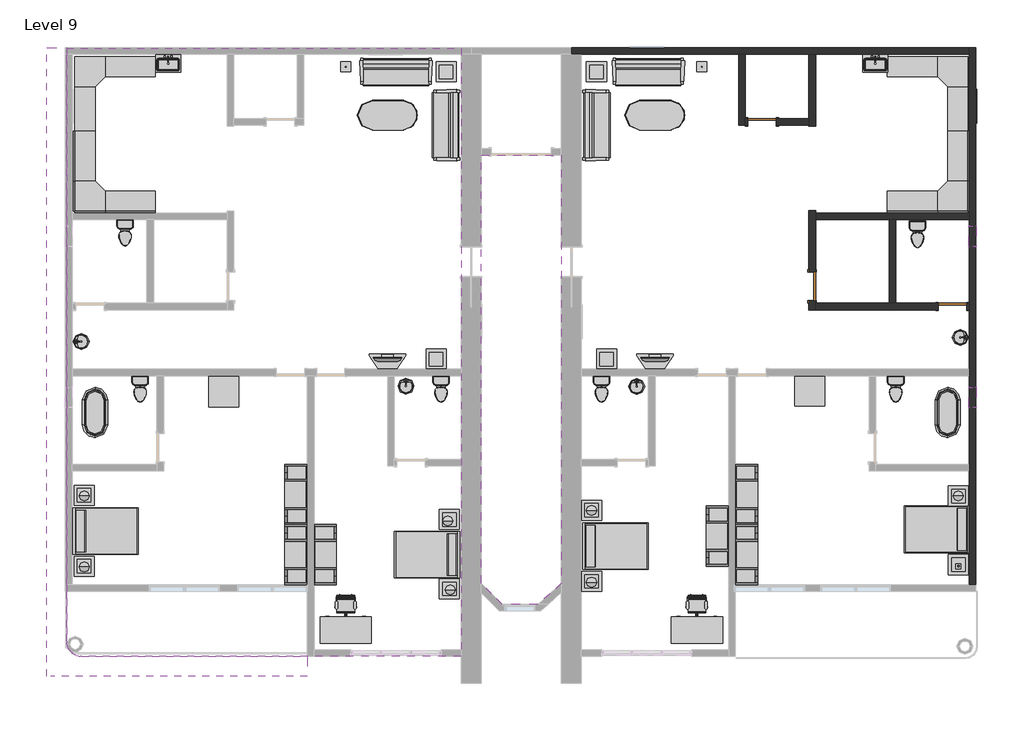
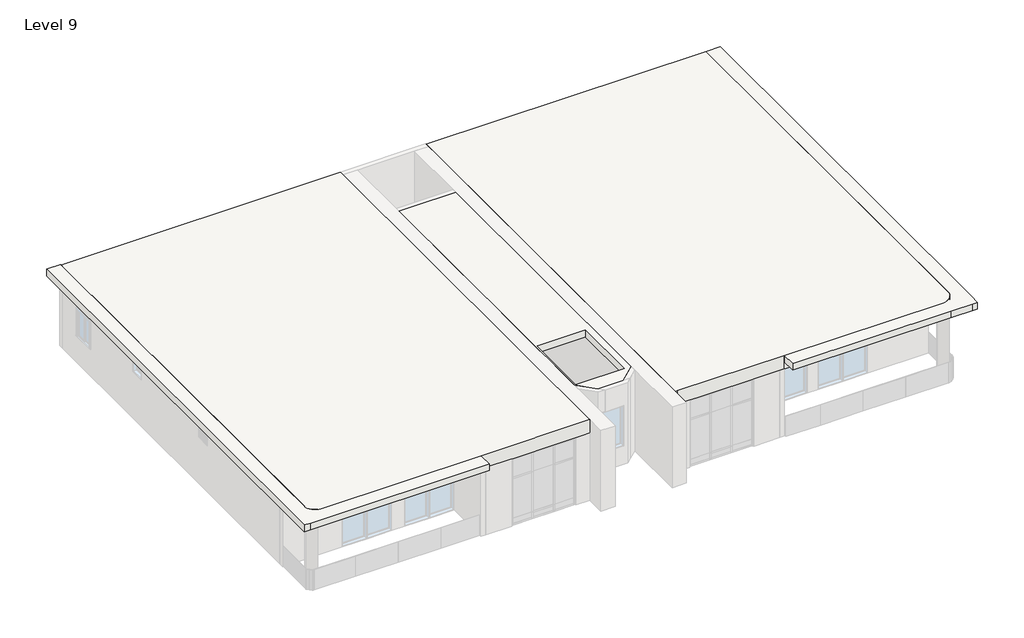
# One storey, part 3 of 3: 42 furniture elements, 14 flow terminals, 10 light fixtures, 9 walls, 3 doors, 3 slabs, 3 windows.
"""IFC4 building model written with IfcOpenShell, lengths in millimetres."""

from ifc_helpers import new_model, si_unit, point, frame, frame_2d, origin, place, context, project, spatial, polyline, circle_curve, trimmed, segment, composite_curve, outline, extrude, faceted_brep, transform, mapped, element, save
from components import door_2703ae13, door_10fd3a06, flow_terminal_38af2918, flow_terminal_d49f872f, toilet_domestic_3d_toilet_domestic_3d_f7549cf7, toilet_domestic_3d_toilet_domestic_3d_183bbd19, flow_terminal_b374fae2, furniture_07436f11, furniture_096e7f55, chair_task_arms_chair_task_arms_fa5a08ef, furniture_072f6425, furniture_cf0b6580, furniture_aff9b2fb, furniture_56245f3a, tv_stand_tv_stand_6ce107e5, furniture_b5c51a22, furniture_2c34a4f9, furniture_4d44e21c, furniture_45e3acac, light_fixture_100w_120v_8564026f, table_lamp_hemispheric_60w_120v_02721d88, window_0038ecf3, window_54100e87

model = new_model("IFC4")

# Units and contexts
model_context = context("Model", 3, world=origin())
ifc_project = project(units=[si_unit("LENGTHUNIT", "METRE", prefix="MILLI")], contexts=[model_context])

# Site, building, storey
site = spatial("IfcSite", under=ifc_project)
building = spatial("IfcBuilding", under=site)
storey = spatial("IfcBuildingStorey", under=building, Name="Level 9", Elevation=29260.8)

# Doors
placement = place(None, origin())
door_shape = door_2703ae13(model_context)
element("IfcDoor", 1, ObjectType="Door-Single-Panel.0001 : 34\" x 80\"", at=placement, inside=storey, context=model_context, shape_type="MappedRepresentation", body=[
    mapped(door_shape, transform((2522.0012296, 9464.0758558, 29260.8), x_axis=(-1.0, 0.0, 0.0), y_axis=(0.0, -1.0, 0.0), z_axis=(0.0, 0.0, 1.0))),
])
door_2_shape = door_10fd3a06(model_context)
element("IfcDoor", 2, ObjectType="Door-Single-Panel.0001 : 34\" x 80\"", at=placement, inside=storey, context=model_context, shape_type="MappedRepresentation", body=[
    mapped(door_2_shape, transform((8313.2012296, 3850.6758558, 29260.8), x_axis=(1.0, 0.0, 0.0), y_axis=(0.0, 1.0, 0.0), z_axis=(0.0, 0.0, 1.0))),
])
element("IfcDoor", 3, ObjectType="Door-Single-Panel.0001 : 34\" x 80\"", at=placement, inside=storey, context=model_context, shape_type="MappedRepresentation", body=[
    mapped(door_2_shape, transform((4046.0012296, 4460.2758558, 29260.8), x_axis=(0.0, -1.0, 0.0), y_axis=(1.0, 0.0, 0.0), z_axis=(0.0, 0.0, 1.0))),
])

# Flow terminals
flow_terminal_shape = flow_terminal_38af2918(model_context)
element("IfcFlowTerminal", 4, ObjectType="Sink Kitchen-Single : 30\" x 21\"", at=placement, inside=storey, context=model_context, shape_type="MappedRepresentation", body=[
    mapped(flow_terminal_shape, transform((-15540.388011, 11239.7304546, 29260.8), x_axis=(1.0, 0.0, 0.0), y_axis=(0.0, 1.0, 0.0), z_axis=(0.0, 0.0, 1.0))),
])
element("IfcFlowTerminal", 5, ObjectType="Sink Kitchen-Single : 30\" x 21\"", at=placement, inside=storey, context=model_context, shape_type="MappedRepresentation", body=[
    mapped(flow_terminal_shape, transform((5948.011989, 11239.7304546, 29260.8), x_axis=(1.0, 0.0, 0.0), y_axis=(0.0, 1.0, 0.0), z_axis=(0.0, 0.0, 1.0))),
])
flow_terminal_2_shape = flow_terminal_d49f872f(model_context)
element("IfcFlowTerminal", 6, ObjectType="Sink Vanity-Round : 19\" x 19\"", at=placement, inside=storey, context=model_context, shape_type="MappedRepresentation", body=[
    mapped(flow_terminal_2_shape, transform((-18084.6070794, 2687.2241152, 29260.8), x_axis=(0.0, 1.0, 0.0), y_axis=(-1.0, 0.0, 0.0), z_axis=(0.0, 0.0, 1.0))),
])
element("IfcFlowTerminal", 7, ObjectType="Sink Vanity-Round : 19\" x 19\"", at=placement, inside=storey, context=model_context, shape_type="MappedRepresentation", body=[
    mapped(flow_terminal_2_shape, transform((8462.2249463, 3007.5275963, 29260.8), x_axis=(0.0, -1.0, 0.0), y_axis=(1.0, 0.0, 0.0), z_axis=(0.0, 0.0, 1.0))),
])
element("IfcFlowTerminal", 8, ObjectType="Sink Vanity-Round : 19\" x 19\"", at=placement, inside=storey, context=model_context, shape_type="MappedRepresentation", body=[
    mapped(flow_terminal_2_shape, transform((-8395.050511, 1341.8921141, 29260.8), x_axis=(1.0, 0.0, 0.0), y_axis=(0.0, 1.0, 0.0), z_axis=(0.0, 0.0, 1.0))),
])
element("IfcFlowTerminal", 9, ObjectType="Sink Vanity-Round : 19\" x 19\"", at=placement, inside=storey, context=model_context, shape_type="MappedRepresentation", body=[
    mapped(flow_terminal_2_shape, transform((-1384.650511, 1331.0855344, 29260.8), x_axis=(1.0, 0.0, 0.0), y_axis=(0.0, 1.0, 0.0), z_axis=(0.0, 0.0, 1.0))),
])
toilet_domestic_3d_toilet_domestic_3d_shape = toilet_domestic_3d_toilet_domestic_3d_f7549cf7(model_context)
toilet_domestic_3d_toilet_domestic_3d_2_shape = toilet_domestic_3d_toilet_domestic_3d_183bbd19(model_context)
element("IfcFlowTerminal", 10, ObjectType="Toilet-Domestic-3D : Toilet-Domestic-3D", at=placement, inside=storey, context=model_context, shape_type="MappedRepresentation", body=[
    mapped(toilet_domestic_3d_toilet_domestic_3d_shape, transform((6586.0012296, 1247.7798284, 29260.8), x_axis=(1.0, 0.0, 0.0), y_axis=(0.0, 1.0, 0.0), z_axis=(0.0, 0.0, 1.0))),
    mapped(toilet_domestic_3d_toilet_domestic_3d_2_shape, transform((6586.0012296, 1247.7798284, 29260.8), x_axis=(1.0, 0.0, 0.0), y_axis=(0.0, 1.0, 0.0), z_axis=(0.0, 0.0, 1.0))),
])
element("IfcFlowTerminal", 11, ObjectType="Toilet-Domestic-3D : Toilet-Domestic-3D", at=placement, inside=storey, context=model_context, shape_type="MappedRepresentation", body=[
    mapped(toilet_domestic_3d_toilet_domestic_3d_shape, transform((-2354.7987704, 1247.7798284, 29260.8), x_axis=(1.0, 0.0, 0.0), y_axis=(0.0, 1.0, 0.0), z_axis=(0.0, 0.0, 1.0))),
    mapped(toilet_domestic_3d_toilet_domestic_3d_2_shape, transform((-2354.7987704, 1247.7798284, 29260.8), x_axis=(1.0, 0.0, 0.0), y_axis=(0.0, 1.0, 0.0), z_axis=(0.0, 0.0, 1.0))),
])
element("IfcFlowTerminal", 12, ObjectType="Toilet-Domestic-3D : Toilet-Domestic-3D", at=placement, inside=storey, context=model_context, shape_type="MappedRepresentation", body=[
    mapped(toilet_domestic_3d_toilet_domestic_3d_shape, transform((-16375.5987704, 1247.7798284, 29260.8), x_axis=(1.0, 0.0, 0.0), y_axis=(0.0, 1.0, 0.0), z_axis=(0.0, 0.0, 1.0))),
    mapped(toilet_domestic_3d_toilet_domestic_3d_2_shape, transform((-16375.5987704, 1247.7798284, 29260.8), x_axis=(1.0, 0.0, 0.0), y_axis=(0.0, 1.0, 0.0), z_axis=(0.0, 0.0, 1.0))),
])
element("IfcFlowTerminal", 13, ObjectType="Toilet-Domestic-3D : Toilet-Domestic-3D", at=placement, inside=storey, context=model_context, shape_type="MappedRepresentation", body=[
    mapped(toilet_domestic_3d_toilet_domestic_3d_shape, transform((-16832.7987704, 5997.5798284, 29260.8), x_axis=(1.0, 0.0, 0.0), y_axis=(0.0, 1.0, 0.0), z_axis=(0.0, 0.0, 1.0))),
    mapped(toilet_domestic_3d_toilet_domestic_3d_2_shape, transform((-16832.7987704, 5997.5798284, 29260.8), x_axis=(1.0, 0.0, 0.0), y_axis=(0.0, 1.0, 0.0), z_axis=(0.0, 0.0, 1.0))),
])
element("IfcFlowTerminal", 14, ObjectType="Toilet-Domestic-3D : Toilet-Domestic-3D", at=placement, inside=storey, context=model_context, shape_type="MappedRepresentation", body=[
    mapped(toilet_domestic_3d_toilet_domestic_3d_shape, transform((7246.4012296, 5946.7798284, 29260.8), x_axis=(1.0, 0.0, 0.0), y_axis=(0.0, 1.0, 0.0), z_axis=(0.0, 0.0, 1.0))),
    mapped(toilet_domestic_3d_toilet_domestic_3d_2_shape, transform((7246.4012296, 5946.7798284, 29260.8), x_axis=(1.0, 0.0, 0.0), y_axis=(0.0, 1.0, 0.0), z_axis=(0.0, 0.0, 1.0))),
])
element("IfcFlowTerminal", 15, ObjectType="Toilet-Domestic-3D : Toilet-Domestic-3D", at=placement, inside=storey, context=model_context, shape_type="MappedRepresentation", body=[
    mapped(toilet_domestic_3d_toilet_domestic_3d_shape, transform((-7231.5987704, 1247.7798284, 29260.8), x_axis=(1.0, 0.0, 0.0), y_axis=(0.0, 1.0, 0.0), z_axis=(0.0, 0.0, 1.0))),
    mapped(toilet_domestic_3d_toilet_domestic_3d_2_shape, transform((-7231.5987704, 1247.7798284, 29260.8), x_axis=(1.0, 0.0, 0.0), y_axis=(0.0, 1.0, 0.0), z_axis=(0.0, 0.0, 1.0))),
])
flow_terminal_3_shape = flow_terminal_b374fae2(model_context)
element("IfcFlowTerminal", 16, ObjectType="Tub-Free Standing-3D : 30\" x 60\"", at=placement, inside=storey, context=model_context, shape_type="MappedRepresentation", body=[
    mapped(flow_terminal_3_shape, transform((-17747.1987704, 624.8758558, 29260.8), x_axis=(1.0, 0.0, 0.0), y_axis=(0.0, 1.0, 0.0), z_axis=(0.0, 0.0, 1.0))),
])
element("IfcFlowTerminal", 17, ObjectType="Tub-Free Standing-3D : 30\" x 60\"", at=placement, inside=storey, context=model_context, shape_type="MappedRepresentation", body=[
    mapped(flow_terminal_3_shape, transform((8160.8012296, 624.8758558, 29260.8), x_axis=(1.0, 0.0, 0.0), y_axis=(0.0, 1.0, 0.0), z_axis=(0.0, 0.0, 1.0))),
])

# Furniture
furniture_shape = furniture_07436f11(model_context)
element("IfcFurniture", 18, ObjectType="96\" x 96\"", at=placement, inside=storey, context=model_context, shape_type="MappedRepresentation", body=[
    mapped(furniture_shape, transform((-18275.8670182, 11991.0988634, 29260.8), x_axis=(1.0, 0.0, 0.0), y_axis=(0.0, 1.0, 0.0), z_axis=(0.0, 0.0, 1.0))),
])
element("IfcFurniture", 19, ObjectType="96\" x 96\"", at=placement, inside=storey, context=model_context, shape_type="MappedRepresentation", body=[
    mapped(furniture_shape, transform((9316.2242372, 11364.3441035, 29260.8), x_axis=(0.0, -1.0, 0.0), y_axis=(1.0, 0.0, 0.0), z_axis=(0.0, 0.0, 1.0))),
])
furniture_2_shape = furniture_096e7f55(model_context)
element("IfcFurniture", 20, ObjectType="Bed-Shaker : Double 56\" x 78\"", at=placement, inside=storey, context=model_context, shape_type="MappedRepresentation", body=[
    mapped(furniture_2_shape, transform((-18407.5987704, -2962.8741442, 29260.8), x_axis=(0.0, 1.0, 0.0), y_axis=(-1.0, 0.0, 0.0), z_axis=(0.0, 0.0, 1.0))),
])
element("IfcFurniture", 21, ObjectType="Bed-Shaker : Double 56\" x 78\"", at=placement, inside=storey, context=model_context, shape_type="MappedRepresentation", body=[
    mapped(furniture_2_shape, transform((-6672.7987704, -3712.1741442, 29260.8), x_axis=(0.0, -1.0, 0.0), y_axis=(1.0, 0.0, 0.0), z_axis=(0.0, 0.0, 1.0))),
])
element("IfcFurniture", 22, ObjectType="Bed-Shaker : Double 56\" x 78\"", at=placement, inside=storey, context=model_context, shape_type="MappedRepresentation", body=[
    mapped(furniture_2_shape, transform((-2913.5987704, -3420.0741442, 29260.8), x_axis=(0.0, 1.0, 0.0), y_axis=(-1.0, 0.0, 0.0), z_axis=(0.0, 0.0, 1.0))),
])
element("IfcFurniture", 23, ObjectType="Bed-Shaker : Double 56\" x 78\"", at=placement, inside=storey, context=model_context, shape_type="MappedRepresentation", body=[
    mapped(furniture_2_shape, transform((8821.2012296, -2950.1741442, 29260.8), x_axis=(0.0, -1.0, 0.0), y_axis=(1.0, 0.0, 0.0), z_axis=(0.0, 0.0, 1.0))),
])
chair_task_arms_chair_task_arms_shape = chair_task_arms_chair_task_arms_fa5a08ef(model_context)
element("IfcFurniture", 24, ObjectType="Chair-Task Arms : Chair-Task Arms", at=placement, inside=storey, context=model_context, shape_type="MappedRepresentation", body=[
    mapped(chair_task_arms_chair_task_arms_shape, transform((681.7920493, -5184.3566833, 29260.8), x_axis=(-1.0, 0.0, 0.0), y_axis=(0.0, -1.0, 0.0), z_axis=(0.0, 0.0, 1.0))),
])
element("IfcFurniture", 25, ObjectType="Chair-Task Arms : Chair-Task Arms", at=placement, inside=storey, context=model_context, shape_type="MappedRepresentation", body=[
    mapped(chair_task_arms_chair_task_arms_shape, transform((-9986.2079507, -5184.3566833, 29260.8), x_axis=(-1.0, 0.0, 0.0), y_axis=(0.0, -1.0, 0.0), z_axis=(0.0, 0.0, 1.0))),
])
furniture_3_shape = furniture_072f6425(model_context)
element("IfcFurniture", 26, ObjectType="Desk : 60\" x 30\"", at=placement, inside=storey, context=model_context, shape_type="MappedRepresentation", body=[
    mapped(furniture_3_shape, transform((-10889.1987704, -6371.702585, 29260.8), x_axis=(1.0, 0.0, 0.0), y_axis=(0.0, 1.0, 0.0), z_axis=(0.0, 0.0, 1.0))),
])
element("IfcFurniture", 27, ObjectType="Desk : 60\" x 30\"", at=placement, inside=storey, context=model_context, shape_type="MappedRepresentation", body=[
    mapped(furniture_3_shape, transform((-221.1987704, -6371.702585, 29260.8), x_axis=(1.0, 0.0, 0.0), y_axis=(0.0, 1.0, 0.0), z_axis=(0.0, 0.0, 1.0))),
])
furniture_4_shape = furniture_cf0b6580(model_context)
element("IfcFurniture", 28, ObjectType="Entertainment Center : 72\" x 72\" x 24\"", at=placement, inside=storey, context=model_context, shape_type="MappedRepresentation", body=[
    mapped(furniture_4_shape, transform((1607.6012296, -3134.3241442, 29260.8), x_axis=(0.0, -1.0, 0.0), y_axis=(1.0, 0.0, 0.0), z_axis=(0.0, 0.0, 1.0))),
])
element("IfcFurniture", 29, ObjectType="Entertainment Center : 72\" x 72\" x 24\"", at=placement, inside=storey, context=model_context, shape_type="MappedRepresentation", body=[
    mapped(furniture_4_shape, transform((1607.6012296, -3693.1241442, 29260.8), x_axis=(0.0, 1.0, 0.0), y_axis=(-1.0, 0.0, 0.0), z_axis=(0.0, 0.0, 1.0))),
])
element("IfcFurniture", 30, ObjectType="Entertainment Center : 72\" x 72\" x 24\"", at=placement, inside=storey, context=model_context, shape_type="MappedRepresentation", body=[
    mapped(furniture_4_shape, transform((1607.6012296, -1864.3241442, 29260.8), x_axis=(0.0, 1.0, 0.0), y_axis=(-1.0, 0.0, 0.0), z_axis=(0.0, 0.0, 1.0))),
])
element("IfcFurniture", 31, ObjectType="Entertainment Center : 72\" x 72\" x 24\"", at=placement, inside=storey, context=model_context, shape_type="MappedRepresentation", body=[
    mapped(furniture_4_shape, transform((-11193.9987704, -3693.1241442, 29260.8), x_axis=(0.0, -1.0, 0.0), y_axis=(1.0, 0.0, 0.0), z_axis=(0.0, 0.0, 1.0))),
])
element("IfcFurniture", 32, ObjectType="Entertainment Center : 72\" x 72\" x 24\"", at=placement, inside=storey, context=model_context, shape_type="MappedRepresentation", body=[
    mapped(furniture_4_shape, transform((-11193.9987704, -1864.3241442, 29260.8), x_axis=(0.0, -1.0, 0.0), y_axis=(1.0, 0.0, 0.0), z_axis=(0.0, 0.0, 1.0))),
])
element("IfcFurniture", 33, ObjectType="Entertainment Center : 72\" x 72\" x 24\"", at=placement, inside=storey, context=model_context, shape_type="MappedRepresentation", body=[
    mapped(furniture_4_shape, transform((-11193.9987704, -3693.1241442, 29260.8), x_axis=(0.0, 1.0, 0.0), y_axis=(-1.0, 0.0, 0.0), z_axis=(0.0, 0.0, 1.0))),
])
furniture_5_shape = furniture_aff9b2fb(model_context)
element("IfcFurniture", 34, ObjectType="Sofa-Pensi : 84\"", at=placement, inside=storey, context=model_context, shape_type="MappedRepresentation", body=[
    mapped(furniture_5_shape, transform((-8881.8050204, 10710.9660197, 29260.8), x_axis=(1.0, 0.0, 0.0), y_axis=(0.0, 1.0, 0.0), z_axis=(0.0, 0.0, 1.0))),
])
element("IfcFurniture", 35, ObjectType="Sofa-Pensi : 84\"", at=placement, inside=storey, context=model_context, shape_type="MappedRepresentation", body=[
    mapped(furniture_5_shape, transform((-7356.3086065, 9641.0821058, 29260.8), x_axis=(0.0, -1.0, 0.0), y_axis=(1.0, 0.0, 0.0), z_axis=(0.0, 0.0, 1.0))),
])
element("IfcFurniture", 36, ObjectType="Sofa-Pensi : 84\"", at=placement, inside=storey, context=model_context, shape_type="MappedRepresentation", body=[
    mapped(furniture_5_shape, transform((-2230.0889343, 9083.8696058, 29260.8), x_axis=(0.0, 1.0, 0.0), y_axis=(-1.0, 0.0, 0.0), z_axis=(0.0, 0.0, 1.0))),
])
element("IfcFurniture", 37, ObjectType="Sofa-Pensi : 84\"", at=placement, inside=storey, context=model_context, shape_type="MappedRepresentation", body=[
    mapped(furniture_5_shape, transform((-1211.0050204, 10710.9660197, 29260.8), x_axis=(1.0, 0.0, 0.0), y_axis=(0.0, 1.0, 0.0), z_axis=(0.0, 0.0, 1.0))),
])
furniture_6_shape = furniture_56245f3a(model_context)
element("IfcFurniture", 38, ObjectType="TV - Flat Screen : 32\"", at=placement, inside=storey, context=model_context, shape_type="MappedRepresentation", body=[
    mapped(furniture_6_shape, transform((-8861.1432846, 2232.8144794, 30175.2), x_axis=(-1.0, 0.0, 0.0), y_axis=(0.0, -1.0, 0.0), z_axis=(0.0, 0.0, 1.0))),
])
element("IfcFurniture", 39, ObjectType="TV - Flat Screen : 32\"", at=placement, inside=storey, context=model_context, shape_type="MappedRepresentation", body=[
    mapped(furniture_6_shape, transform((-733.1432846, 2232.8144794, 30175.2), x_axis=(-1.0, 0.0, 0.0), y_axis=(0.0, -1.0, 0.0), z_axis=(0.0, 0.0, 1.0))),
])
tv_stand_tv_stand_shape = tv_stand_tv_stand_6ce107e5(model_context)
element("IfcFurniture", 40, ObjectType="TV Stand : TV Stand", at=placement, inside=storey, context=model_context, shape_type="MappedRepresentation", body=[
    mapped(tv_stand_tv_stand_shape, transform((-8732.0107683, 1945.6758558, 29260.8), x_axis=(-1.0, 0.0, 0.0), y_axis=(0.0, -1.0, 0.0), z_axis=(0.0, 0.0, 1.0))),
])
element("IfcFurniture", 41, ObjectType="TV Stand : TV Stand", at=placement, inside=storey, context=model_context, shape_type="MappedRepresentation", body=[
    mapped(tv_stand_tv_stand_shape, transform((-604.0107683, 1945.6758558, 29260.8), x_axis=(-1.0, 0.0, 0.0), y_axis=(0.0, -1.0, 0.0), z_axis=(0.0, 0.0, 1.0))),
])
furniture_7_shape = furniture_b5c51a22(model_context)
element("IfcFurniture", 42, ObjectType="Table-Coffee : 24\" x 24\" x 24\"", at=placement, inside=storey, context=model_context, shape_type="MappedRepresentation", body=[
    mapped(furniture_7_shape, transform((-7097.4645371, 10892.864778, 29260.8), x_axis=(1.0, 0.0, 0.0), y_axis=(0.0, 1.0, 0.0), z_axis=(0.0, 0.0, 1.0))),
])
element("IfcFurniture", 43, ObjectType="Table-Coffee : 24\" x 24\" x 24\"", at=placement, inside=storey, context=model_context, shape_type="MappedRepresentation", body=[
    mapped(furniture_7_shape, transform((-2525.4645371, 10892.864778, 29260.8), x_axis=(1.0, 0.0, 0.0), y_axis=(0.0, 1.0, 0.0), z_axis=(0.0, 0.0, 1.0))),
])
element("IfcFurniture", 44, ObjectType="Table-Coffee : 24\" x 24\" x 24\"", at=placement, inside=storey, context=model_context, shape_type="MappedRepresentation", body=[
    mapped(furniture_7_shape, transform((-7402.2645371, 2155.264778, 29260.8), x_axis=(1.0, 0.0, 0.0), y_axis=(0.0, 1.0, 0.0), z_axis=(0.0, 0.0, 1.0))),
])
element("IfcFurniture", 45, ObjectType="Table-Coffee : 24\" x 24\" x 24\"", at=placement, inside=storey, context=model_context, shape_type="MappedRepresentation", body=[
    mapped(furniture_7_shape, transform((-2220.6645371, 2155.264778, 29260.8), x_axis=(1.0, 0.0, 0.0), y_axis=(0.0, 1.0, 0.0), z_axis=(0.0, 0.0, 1.0))),
])
element("IfcFurniture", 46, ObjectType="Table-Coffee : 24\" x 24\" x 24\"", at=placement, inside=storey, context=model_context, shape_type="MappedRepresentation", body=[
    mapped(furniture_7_shape, transform((-2677.8645371, -4601.135222, 29260.8), x_axis=(1.0, 0.0, 0.0), y_axis=(0.0, 1.0, 0.0), z_axis=(0.0, 0.0, 1.0))),
])
element("IfcFurniture", 47, ObjectType="Table-Coffee : 24\" x 24\" x 24\"", at=placement, inside=storey, context=model_context, shape_type="MappedRepresentation", body=[
    mapped(furniture_7_shape, transform((-18095.6645371, -4143.935222, 29260.8), x_axis=(1.0, 0.0, 0.0), y_axis=(0.0, 1.0, 0.0), z_axis=(0.0, 0.0, 1.0))),
])
element("IfcFurniture", 48, ObjectType="Table-Coffee : 24\" x 24\" x 24\"", at=placement, inside=storey, context=model_context, shape_type="MappedRepresentation", body=[
    mapped(furniture_7_shape, transform((-18095.6645371, -1984.935222, 29260.8), x_axis=(1.0, 0.0, 0.0), y_axis=(0.0, 1.0, 0.0), z_axis=(0.0, 0.0, 1.0))),
])
element("IfcFurniture", 49, ObjectType="Table-Coffee : 24\" x 24\" x 24\"", at=placement, inside=storey, context=model_context, shape_type="MappedRepresentation", body=[
    mapped(furniture_7_shape, transform((-2677.8645371, -2442.135222, 29260.8), x_axis=(1.0, 0.0, 0.0), y_axis=(0.0, 1.0, 0.0), z_axis=(0.0, 0.0, 1.0))),
])
element("IfcFurniture", 50, ObjectType="Table-Coffee : 24\" x 24\" x 24\"", at=placement, inside=storey, context=model_context, shape_type="MappedRepresentation", body=[
    mapped(furniture_7_shape, transform((8472.7354629, -4093.135222, 29260.8), x_axis=(1.0, 0.0, 0.0), y_axis=(0.0, 1.0, 0.0), z_axis=(0.0, 0.0, 1.0))),
])
element("IfcFurniture", 51, ObjectType="Table-Coffee : 24\" x 24\" x 24\"", at=placement, inside=storey, context=model_context, shape_type="MappedRepresentation", body=[
    mapped(furniture_7_shape, transform((8472.7354629, -2010.335222, 29260.8), x_axis=(1.0, 0.0, 0.0), y_axis=(0.0, 1.0, 0.0), z_axis=(0.0, 0.0, 1.0))),
])
element("IfcFurniture", 52, ObjectType="Table-Coffee : 24\" x 24\" x 24\"", at=placement, inside=storey, context=model_context, shape_type="MappedRepresentation", body=[
    mapped(furniture_7_shape, transform((-6995.8645371, -4832.0414601, 29260.8), x_axis=(1.0, 0.0, 0.0), y_axis=(0.0, 1.0, 0.0), z_axis=(0.0, 0.0, 1.0))),
])
element("IfcFurniture", 53, ObjectType="Table-Coffee : 24\" x 24\" x 24\"", at=placement, inside=storey, context=model_context, shape_type="MappedRepresentation", body=[
    mapped(furniture_7_shape, transform((-6995.8645371, -2723.8414601, 29260.8), x_axis=(1.0, 0.0, 0.0), y_axis=(0.0, 1.0, 0.0), z_axis=(0.0, 0.0, 1.0))),
])
furniture_8_shape = furniture_2c34a4f9(model_context)
element("IfcFurniture", 54, ObjectType="Table-Dining Oval : 36\" x 72\"", at=placement, inside=storey, context=model_context, shape_type="MappedRepresentation", body=[
    mapped(furniture_8_shape, transform((-8455.3790983, 10025.3742164, 29260.8), x_axis=(1.0, 0.0, 0.0), y_axis=(0.0, 1.0, 0.0), z_axis=(0.0, 0.0, 1.0))),
])
element("IfcFurniture", 55, ObjectType="Table-Dining Oval : 36\" x 72\"", at=placement, inside=storey, context=model_context, shape_type="MappedRepresentation", body=[
    mapped(furniture_8_shape, transform((-327.3790983, 10025.3742164, 29260.8), x_axis=(1.0, 0.0, 0.0), y_axis=(0.0, 1.0, 0.0), z_axis=(0.0, 0.0, 1.0))),
])
furniture_9_shape = furniture_4d44e21c(model_context)
element("IfcFurniture", 56, ObjectType="Table-Rectangular : 36\" x 36\"", at=placement, inside=storey, context=model_context, shape_type="MappedRepresentation", body=[
    mapped(furniture_9_shape, transform((-13835.5987704, 1259.8758558, 29260.8), x_axis=(1.0, 0.0, 0.0), y_axis=(0.0, 1.0, 0.0), z_axis=(0.0, 0.0, 1.0))),
])
element("IfcFurniture", 57, ObjectType="Table-Rectangular : 36\" x 36\"", at=placement, inside=storey, context=model_context, shape_type="MappedRepresentation", body=[
    mapped(furniture_9_shape, transform((3969.8012296, 1285.2758558, 29260.8), x_axis=(1.0, 0.0, 0.0), y_axis=(0.0, 1.0, 0.0), z_axis=(0.0, 0.0, 1.0))),
])
furniture_10_shape = furniture_45e3acac(model_context)
element("IfcFurniture", 58, ObjectType="Work Station Cubicle : 96\" x 96\"", at=placement, inside=storey, context=model_context, shape_type="MappedRepresentation", body=[
    mapped(furniture_10_shape, transform((-18902.621778, 6827.207608, 29260.8), x_axis=(0.0, 1.0, 0.0), y_axis=(-1.0, 0.0, 0.0), z_axis=(0.0, 0.0, 1.0))),
])
element("IfcFurniture", 59, ObjectType="Work Station Cubicle : 96\" x 96\"", at=placement, inside=storey, context=model_context, shape_type="MappedRepresentation", body=[
    mapped(furniture_10_shape, transform((8689.4694774, 6200.4528481, 29260.8), x_axis=(-1.0, 0.0, 0.0), y_axis=(0.0, -1.0, 0.0), z_axis=(0.0, 0.0, 1.0))),
])

# Light fixtures
light_fixture_100w_120v_shape = light_fixture_100w_120v_8564026f(model_context)
element("IfcLightFixture", 60, ObjectType="100W - 120V", at=placement, inside=storey, context=model_context, shape_type="MappedRepresentation", body=[
    mapped(light_fixture_100w_120v_shape, transform((-10127.1987704, 11140.4758558, 29260.8), x_axis=(1.0, 0.0, 0.0), y_axis=(0.0, 1.0, 0.0), z_axis=(0.0, 0.0, 1.0))),
])
element("IfcLightFixture", 61, ObjectType="100W - 120V", at=placement, inside=storey, context=model_context, shape_type="MappedRepresentation", body=[
    mapped(light_fixture_100w_120v_shape, transform((693.2012296, 11140.4758558, 29260.8), x_axis=(1.0, 0.0, 0.0), y_axis=(0.0, 1.0, 0.0), z_axis=(0.0, 0.0, 1.0))),
])
table_lamp_hemispheric_60w_120v_shape = table_lamp_hemispheric_60w_120v_02721d88(model_context)
element("IfcLightFixture", 62, ObjectType="Table Lamp - Hemispheric : 60W - 120V", at=placement, inside=storey, context=model_context, shape_type="MappedRepresentation", body=[
    mapped(table_lamp_hemispheric_60w_120v_shape, transform((-18077.3987704, -1915.1241442, 29870.4), x_axis=(1.0, 0.0, 0.0), y_axis=(0.0, 1.0, 0.0), z_axis=(0.0, 0.0, 1.0))),
])
element("IfcLightFixture", 63, ObjectType="Table Lamp - Hemispheric : 60W - 120V", at=placement, inside=storey, context=model_context, shape_type="MappedRepresentation", body=[
    mapped(table_lamp_hemispheric_60w_120v_shape, transform((-7028.3987704, -2666.7303823, 29870.4), x_axis=(1.0, 0.0, 0.0), y_axis=(0.0, 1.0, 0.0), z_axis=(0.0, 0.0, 1.0))),
])
element("IfcLightFixture", 64, ObjectType="Table Lamp - Hemispheric : 60W - 120V", at=placement, inside=storey, context=model_context, shape_type="MappedRepresentation", body=[
    mapped(table_lamp_hemispheric_60w_120v_shape, transform((-2659.5987704, -2346.9241442, 29870.4), x_axis=(1.0, 0.0, 0.0), y_axis=(0.0, 1.0, 0.0), z_axis=(0.0, 0.0, 1.0))),
])
element("IfcLightFixture", 65, ObjectType="Table Lamp - Hemispheric : 60W - 120V", at=placement, inside=storey, context=model_context, shape_type="MappedRepresentation", body=[
    mapped(table_lamp_hemispheric_60w_120v_shape, transform((8491.0012296, -4048.7241442, 30175.2), x_axis=(1.0, 0.0, 0.0), y_axis=(0.0, 1.0, 0.0), z_axis=(0.0, 0.0, 1.0))),
])
element("IfcLightFixture", 66, ObjectType="Table Lamp - Hemispheric : 60W - 120V", at=placement, inside=storey, context=model_context, shape_type="MappedRepresentation", body=[
    mapped(table_lamp_hemispheric_60w_120v_shape, transform((8491.0012296, -1915.1241442, 29870.4), x_axis=(1.0, 0.0, 0.0), y_axis=(0.0, 1.0, 0.0), z_axis=(0.0, 0.0, 1.0))),
])
element("IfcLightFixture", 67, ObjectType="Table Lamp - Hemispheric : 60W - 120V", at=placement, inside=storey, context=model_context, shape_type="MappedRepresentation", body=[
    mapped(table_lamp_hemispheric_60w_120v_shape, transform((-2659.5987704, -4531.3241442, 29870.4), x_axis=(1.0, 0.0, 0.0), y_axis=(0.0, 1.0, 0.0), z_axis=(0.0, 0.0, 1.0))),
])
element("IfcLightFixture", 68, ObjectType="Table Lamp - Hemispheric : 60W - 120V", at=placement, inside=storey, context=model_context, shape_type="MappedRepresentation", body=[
    mapped(table_lamp_hemispheric_60w_120v_shape, transform((-6952.1987704, -4762.2303823, 29870.4), x_axis=(1.0, 0.0, 0.0), y_axis=(0.0, 1.0, 0.0), z_axis=(0.0, 0.0, 1.0))),
])
element("IfcLightFixture", 69, ObjectType="Table Lamp - Hemispheric : 60W - 120V", at=placement, inside=storey, context=model_context, shape_type="MappedRepresentation", body=[
    mapped(table_lamp_hemispheric_60w_120v_shape, transform((-18077.3987704, -4074.1241442, 29870.4), x_axis=(1.0, 0.0, 0.0), y_axis=(0.0, 1.0, 0.0), z_axis=(0.0, 0.0, 1.0))),
])

# Slabs
element("IfcSlab", 70, ObjectType="Generic - 12\" cream", at=placement, inside=storey, context=model_context, shape_type="SweptSolid", body=[
    extrude(outline(composite_curve([segment(polyline([(-6621.9987704, 11699.2758558), (-6621.9987704, -6791.9241442), (-11295.5987704, -6791.9241442), (-18153.5987704, -6791.9241442)]), True, "CONTINUOUS"), segment(trimmed(circle_curve(frame_2d((-18153.5987704, -6334.7241442)), 457.2), [point((-18153.5987704, -6791.9241442))], [point((-18610.7987704, -6334.7241442))], False, "CARTESIAN"), True, "CONTINUOUS"), segment(polyline([(-18610.7987704, -6334.7241442), (-18610.7987704, 11699.2758558), (-6621.9987704, 11699.2758558)]), True, "CONTINUOUS")], self_intersect=False)), frame((0.0, 0.0, 32308.8), z_axis=(0.0, 0.0, 1.0), x_axis=(1.0, 0.0, 0.0)), (0.0, 0.0, 1.0), 609.6),
    extrude(outline(composite_curve([segment(trimmed(circle_curve(frame_2d((8511.8043381, -6277.3874522)), 514.536692), [point((9024.4012296, -6322.0241442))], [point((8511.8043381, -6791.9241442))], False, "CARTESIAN"), True, "CONTINUOUS"), segment(polyline([(8511.8043381, -6791.9241442), (1709.2012296, -6791.9241442), (-2862.7987704, -6791.9241442), (-2964.3987704, -6791.9241442), (-2964.3987704, 11699.2758558), (9024.4012296, 11699.2758558), (9024.4012296, -6322.0241442)]), True, "CONTINUOUS")], self_intersect=False)), frame((0.0, 0.0, 32308.8), z_axis=(0.0, 0.0, 1.0), x_axis=(1.0, 0.0, 0.0)), (0.0, 0.0, 1.0), 609.6),
])
element("IfcSlab", 71, ObjectType="Generic - 12\" white", at=placement, inside=storey, context=model_context, shape_type="SweptSolid", body=[
    extrude(outline(composite_curve([segment(polyline([(9634.0012296, 11699.2758558), (9634.0012296, -6931.6241442), (9634.0012296, -7401.5241442), (9430.8012296, -7401.5241442), (8511.8043381, -7401.5241442), (1709.2012296, -7401.5241442), (1709.2012296, -6791.9241442), (8511.8043381, -6791.9241442)]), True, "CONTINUOUS"), segment(trimmed(circle_curve(frame_2d((8511.8043381, -6277.3874522)), 514.536692), [point((8511.8043381, -6791.9241442))], [point((9024.4012296, -6322.0241442))], True, "CARTESIAN"), True, "CONTINUOUS"), segment(polyline([(9024.4012296, -6322.0241442), (9024.4012296, 11699.2758558), (9634.0012296, 11699.2758558)]), True, "CONTINUOUS")], self_intersect=False)), frame((0.0, 0.0, 32613.6), z_axis=(0.0, 0.0, 1.0), x_axis=(1.0, 0.0, 0.0)), (0.0, 0.0, 1.0), 304.8),
    extrude(outline(composite_curve([segment(polyline([(-18610.7987704, 11724.6758558), (-18610.7987704, -6334.7241442)]), True, "CONTINUOUS"), segment(trimmed(circle_curve(frame_2d((-18153.5987704, -6334.7241442)), 457.2), [point((-18610.7987704, -6334.7241442))], [point((-18153.5987704, -6791.9241442))], True, "CARTESIAN"), True, "CONTINUOUS"), segment(polyline([(-18153.5987704, -6791.9241442), (-11295.5987704, -6791.9241442), (-11295.5987704, -7401.5241442), (-18966.3987704, -7401.5241442), (-19220.3987704, -7401.5241442), (-19220.3987704, 11724.6758558), (-18610.7987704, 11724.6758558)]), True, "CONTINUOUS")], self_intersect=False)), frame((0.0, 0.0, 32613.6), z_axis=(0.0, 0.0, 1.0), x_axis=(1.0, 0.0, 0.0)), (0.0, 0.0, 1.0), 304.8),
])
element("IfcSlab", 72, ObjectType="Generic - 12\" white", at=placement, inside=storey, context=model_context, shape_type="SweptSolid", body=[
    extrude(outline(polyline([(-3573.9987704, 8448.0758558), (-3573.9987704, -1691.5549149), (-3573.9987704, -4572.9908503), (-4280.7801413, -5203.302585), (-5374.5362318, -5203.302585), (-6012.3987704, -4565.4400463), (-6012.3987704, -1691.5549149), (-6012.3987704, 8448.0758558), (-3573.9987704, 8448.0758558)]), holes=[polyline([(-5940.8822214, -4561.7549149), (-3870.7822214, -4561.7549149), (-3870.7822214, -1691.5549149), (-5940.8822214, -1691.5549149), (-5940.8822214, -4561.7549149)])]), frame((0.0, 0.0, 32613.6), z_axis=(0.0, 0.0, 1.0), x_axis=(1.0, 0.0, 0.0)), (0.0, 0.0, 1.0), 304.8),
])

# Walls
element("IfcWall", 73, ObjectType="Generic - 8\" cream", at=placement, inside=storey, context=model_context, shape_type="Brep", body=[
    faceted_brep([(8821.2012296, 11724.6758558, 29260.8), (8821.2012296, 11521.4758558, 29260.8), (8821.2012296, 6695.4758558, 29260.8), (8821.2012296, 6492.2758558, 29260.8), (8821.2012296, 3952.2758558, 29260.8), (8821.2012296, 3749.0758558, 29260.8), (8821.2012296, 1945.6758558, 29260.8), (8821.2012296, 1742.4758558, 29260.8), (8821.2012296, -949.9241442, 29260.8), (8821.2012296, -1153.1241442, 29260.8), (8821.2012296, -4607.5241442, 29260.8), (8821.2012296, -4607.5241442, 32308.8), (8821.2012296, -1153.1241442, 32308.8), (8821.2012296, -949.9241442, 32308.8), (8821.2012296, 1742.4758558, 32308.8), (8821.2012296, 1945.6758558, 32308.8), (8821.2012296, 3749.0758558, 32308.8), (8821.2012296, 3952.2758558, 32308.8), (8821.2012296, 6492.2758558, 32308.8), (8821.2012296, 6695.4758558, 32308.8), (8821.2012296, 11521.4758558, 32308.8), (8821.2012296, 11724.6758558, 32308.8), (8821.2012296, 10403.8758558, 30480.0), (8821.2012296, 10403.8758558, 31699.2), (8821.2012296, 9489.4758558, 31699.2), (8821.2012296, 9489.4758558, 30480.0), (8821.2012296, 777.2758558, 32004.0), (8821.2012296, 777.2758558, 31394.4), (8821.2012296, 1386.8758558, 31394.4), (8821.2012296, 1386.8758558, 32004.0), (8821.2012296, 6289.0758558, 31394.4), (8821.2012296, 6289.0758558, 32004.0), (8821.2012296, 5679.4758558, 32004.0), (8821.2012296, 5679.4758558, 31394.4), (9024.4012296, -4607.5241442, 29260.8), (9024.4012296, 11724.6758558, 29260.8), (9024.4012296, 11724.6758558, 32308.8), (9024.4012296, -4607.5241442, 32308.8), (9024.4012296, 10403.8758558, 31699.2), (9024.4012296, 10403.8758558, 30480.0), (9024.4012296, 9489.4758558, 30480.0), (9024.4012296, 9489.4758558, 31699.2), (9024.4012296, 777.2758558, 31394.4), (9024.4012296, 777.2758558, 32004.0), (9024.4012296, 1386.8758558, 32004.0), (9024.4012296, 1386.8758558, 31394.4), (9024.4012296, 6289.0758558, 32004.0), (9024.4012296, 6289.0758558, 31394.4), (9024.4012296, 5679.4758558, 31394.4), (9024.4012296, 5679.4758558, 32004.0)], [[[0, 1, 2, 3, 4, 5, 6, 7, 8, 9, 10, 11, 12, 13, 14, 15, 16, 17, 18, 19, 20, 21], [22, 23, 24, 25], [26, 27, 28, 29], [30, 31, 32, 33]], [[34, 35, 36, 37], [38, 39, 40, 41], [42, 43, 44, 45], [46, 47, 48, 49]], [[10, 9, 8, 7, 6, 5, 4, 3, 2, 1, 0, 35, 34]], [[21, 20, 19, 18, 17, 16, 15, 14, 13, 12, 11, 37, 36]], [[0, 21, 36, 35]], [[11, 10, 34, 37]], [[39, 38, 23, 22]], [[40, 39, 22, 25]], [[41, 40, 25, 24]], [[38, 41, 24, 23]], [[26, 43, 42, 27]], [[27, 42, 45, 28]], [[28, 45, 44, 29]], [[43, 26, 29, 44]], [[46, 31, 30, 47]], [[47, 30, 33, 48]], [[48, 33, 32, 49]], [[31, 46, 49, 32]]]),
])
element("IfcWall", 74, ObjectType="Generic - 8\" cream", at=placement, inside=storey, context=model_context, shape_type="Brep", body=[
    faceted_brep([(3944.4012296, 11521.4758558, 29260.8), (3944.4012296, 9565.6758558, 29260.8), (3944.4012296, 9362.4758558, 29260.8), (3944.4012296, 9337.0758558, 29260.8), (3944.4012296, 9337.0758558, 32308.8), (3944.4012296, 9362.4758558, 32308.8), (3944.4012296, 9565.6758558, 32308.8), (3944.4012296, 11521.4758558, 32308.8), (4147.6012296, 11521.4758558, 29260.8), (4147.6012296, 11521.4758558, 32308.8), (4147.6012296, 9337.0758558, 32308.8), (4147.6012296, 9337.0758558, 29260.8)], [[[0, 1, 2, 3, 4, 5, 6, 7]], [[8, 9, 10, 11]], [[3, 2, 1, 0, 8, 11]], [[4, 3, 11, 10]], [[7, 6, 5, 4, 10, 9]], [[0, 7, 9, 8]]]),
])
element("IfcWall", 75, ObjectType="Generic - 8\" cream", at=placement, inside=storey, context=model_context, shape_type="Brep", body=[
    faceted_brep([(4147.6012296, 6492.2758558, 29260.8), (6382.8012296, 6492.2758558, 29260.8), (6586.0012296, 6492.2758558, 29260.8), (8821.2012296, 6492.2758558, 29260.8), (8821.2012296, 6492.2758558, 32308.8), (6586.0012296, 6492.2758558, 32308.8), (6382.8012296, 6492.2758558, 32308.8), (4147.6012296, 6492.2758558, 32308.8), (4147.6012296, 6695.4758558, 29260.8), (4147.6012296, 6695.4758558, 32308.8), (8821.2012296, 6695.4758558, 32308.8), (8821.2012296, 6695.4758558, 29260.8)], [[[0, 1, 2, 3, 4, 5, 6, 7]], [[8, 9, 10, 11]], [[3, 2, 1, 0, 8, 11]], [[7, 6, 5, 4, 10, 9]], [[0, 7, 9, 8]], [[4, 3, 11, 10]]]),
])
element("IfcWall", 76, ObjectType="Generic - 8\" cream", at=placement, inside=storey, context=model_context, shape_type="Brep", body=[
    faceted_brep([(8821.2012296, 3749.0758558, 32308.8), (4147.6012296, 3749.0758558, 32308.8), (4147.6012296, 3749.0758558, 29260.8), (7881.4012296, 3749.0758558, 29260.8), (7881.4012296, 3749.0758558, 31292.8), (8745.0012296, 3749.0758558, 31292.8), (8745.0012296, 3749.0758558, 29260.8), (8821.2012296, 3749.0758558, 29260.8), (4147.6012296, 3952.2758558, 32308.8), (6382.8012296, 3952.2758558, 32308.8), (6586.0012296, 3952.2758558, 32308.8), (8821.2012296, 3952.2758558, 32308.8), (8821.2012296, 3952.2758558, 29260.8), (8745.0012296, 3952.2758558, 29260.8), (8745.0012296, 3952.2758558, 31292.8), (7881.4012296, 3952.2758558, 31292.8), (7881.4012296, 3952.2758558, 29260.8), (6586.0012296, 3952.2758558, 29260.8), (6382.8012296, 3952.2758558, 29260.8), (4147.6012296, 3952.2758558, 29260.8)], [[[0, 1, 2, 3, 4, 5, 6, 7]], [[8, 9, 10, 11, 12, 13, 14, 15, 16, 17, 18, 19]], [[2, 19, 18, 17, 16, 3]], [[12, 7, 6, 13]], [[1, 0, 11, 10, 9, 8]], [[2, 1, 8, 19]], [[0, 7, 12, 11]], [[5, 14, 13, 6]], [[14, 5, 4, 15]], [[15, 4, 3, 16]]]),
])
element("IfcWall", 77, ObjectType="Generic - 8\" cream", at=placement, inside=storey, context=model_context, shape_type="SweptSolid", body=[
    extrude(outline(polyline([(32308.8, 3944.4012296), (32308.8, 2014.0012296), (29260.8, 2014.0012296), (29260.8, 2090.2012296), (31292.8, 2090.2012296), (31292.8, 2953.8012296), (29260.8, 2953.8012296), (29260.8, 3944.4012296), (32308.8, 3944.4012296)])), frame((0.0, 9362.4758558, 0.0), z_axis=(0.0, 1.0, 0.0), x_axis=(0.0, 0.0, 1.0)), (0.0, 0.0, 1.0), 203.2),
])
element("IfcWall", 78, ObjectType="Generic - 8\" cream", at=placement, inside=storey, context=model_context, shape_type="SweptSolid", body=[
    extrude(outline(polyline([(6382.8012296, 3952.2758558), (6382.8012296, 6492.2758558), (6586.0012296, 6492.2758558), (6586.0012296, 3952.2758558), (6382.8012296, 3952.2758558)])), frame((0.0, 0.0, 29260.8), z_axis=(0.0, 0.0, 1.0), x_axis=(1.0, 0.0, 0.0)), (0.0, 0.0, 1.0), 3048.0),
])
element("IfcWall", 79, ObjectType="Generic - 8\" cream", at=placement, inside=storey, context=model_context, shape_type="Brep", body=[
    faceted_brep([(3944.4012296, 3749.0758558, 32308.8), (3944.4012296, 6771.6758558, 32308.8), (3944.4012296, 6771.6758558, 29260.8), (3944.4012296, 4892.0758558, 29260.8), (3944.4012296, 4892.0758558, 31292.8), (3944.4012296, 4028.4758558, 31292.8), (3944.4012296, 4028.4758558, 29260.8), (3944.4012296, 3749.0758558, 29260.8), (4147.6012296, 6771.6758558, 32308.8), (4147.6012296, 6695.4758558, 32308.8), (4147.6012296, 6492.2758558, 32308.8), (4147.6012296, 3952.2758558, 32308.8), (4147.6012296, 3749.0758558, 32308.8), (4147.6012296, 3749.0758558, 29260.8), (4147.6012296, 3952.2758558, 29260.8), (4147.6012296, 4028.4758558, 29260.8), (4147.6012296, 4028.4758558, 31292.8), (4147.6012296, 4892.0758558, 31292.8), (4147.6012296, 4892.0758558, 29260.8), (4147.6012296, 6492.2758558, 29260.8), (4147.6012296, 6695.4758558, 29260.8), (4147.6012296, 6771.6758558, 29260.8)], [[[0, 1, 2, 3, 4, 5, 6, 7]], [[8, 9, 10, 11, 12, 13, 14, 15, 16, 17, 18, 19, 20, 21]], [[2, 21, 20, 19, 18, 3]], [[13, 7, 6, 15, 14]], [[1, 0, 12, 11, 10, 9, 8]], [[2, 1, 8, 21]], [[0, 7, 13, 12]], [[5, 16, 15, 6]], [[16, 5, 4, 17]], [[17, 4, 3, 18]]]),
])
element("IfcWall", 80, ObjectType="Generic - 8\" cream", at=placement, inside=storey, context=model_context, shape_type="Brep", body=[
    faceted_brep([(-3269.1987704, 11521.4758558, 29260.8), (-2964.3987704, 11521.4758558, 29260.8), (1810.8012296, 11521.4758558, 29260.8), (2014.0012296, 11521.4758558, 29260.8), (3944.4012296, 11521.4758558, 29260.8), (4147.6012296, 11521.4758558, 29260.8), (8821.2012296, 11521.4758558, 29260.8), (8821.2012296, 11521.4758558, 32308.8), (4147.6012296, 11521.4758558, 32308.8), (3944.4012296, 11521.4758558, 32308.8), (2014.0012296, 11521.4758558, 32308.8), (1810.8012296, 11521.4758558, 32308.8), (-2964.3987704, 11521.4758558, 32308.8), (-3269.1987704, 11521.4758558, 32308.8), (-1440.3987704, 11521.4758558, 31699.2), (-525.9987704, 11521.4758558, 31699.2), (-525.9987704, 11521.4758558, 30480.0), (-1440.3987704, 11521.4758558, 30480.0), (-3269.1987704, 11724.6758558, 29260.8), (-3269.1987704, 11724.6758558, 32308.8), (-2964.3987704, 11724.6758558, 32308.8), (8821.2012296, 11724.6758558, 32308.8), (8821.2012296, 11724.6758558, 29260.8), (-1440.3987704, 11724.6758558, 31699.2), (-1440.3987704, 11724.6758558, 30480.0), (-525.9987704, 11724.6758558, 30480.0), (-525.9987704, 11724.6758558, 31699.2)], [[[0, 1, 2, 3, 4, 5, 6, 7, 8, 9, 10, 11, 12, 13], [14, 15, 16, 17]], [[18, 19, 20, 21, 22], [23, 24, 25, 26]], [[6, 5, 4, 3, 2, 1, 0, 18, 22]], [[13, 12, 11, 10, 9, 8, 7, 21, 20, 19]], [[0, 13, 19, 18]], [[7, 6, 22, 21]], [[23, 26, 15, 14]], [[26, 25, 16, 15]], [[25, 24, 17, 16]], [[24, 23, 14, 17]]]),
])
element("IfcWall", 81, ObjectType="Generic - 8\" white", at=placement, inside=storey, context=model_context, shape_type="Brep", body=[
    faceted_brep([(1810.8012296, 11521.4758558, 29260.8), (1810.8012296, 9362.4758558, 29260.8), (1810.8012296, 9362.4758558, 32308.8), (1810.8012296, 11521.4758558, 32308.8), (2014.0012296, 11521.4758558, 29260.8), (2014.0012296, 11521.4758558, 32308.8), (2014.0012296, 9565.6758558, 32308.8), (2014.0012296, 9362.4758558, 32308.8), (2014.0012296, 9362.4758558, 29260.8), (2014.0012296, 9565.6758558, 29260.8)], [[[0, 1, 2, 3]], [[4, 5, 6, 7, 8, 9]], [[1, 0, 4, 9, 8]], [[3, 2, 7, 6, 5]], [[0, 3, 5, 4]], [[2, 1, 8, 7]]]),
])

# Windows
window_shape = window_0038ecf3(model_context)
element("IfcWindow", 82, ObjectType="Louvers with Trim : 24\" x 24\"", at=placement, inside=storey, context=model_context, shape_type="MappedRepresentation", body=[
    mapped(window_shape, transform((8916.4512296, 5984.2758558, 30480.0), x_axis=(0.0, 1.0, 0.0), y_axis=(-1.0, 0.0, 0.0), z_axis=(0.0, 0.0, 1.0))),
])
element("IfcWindow", 83, ObjectType="Louvers with Trim : 24\" x 24\"", at=placement, inside=storey, context=model_context, shape_type="MappedRepresentation", body=[
    mapped(window_shape, transform((8929.1512296, 1082.0758558, 30480.0), x_axis=(0.0, -1.0, 0.0), y_axis=(1.0, 0.0, 0.0), z_axis=(0.0, 0.0, 1.0))),
])
window_2_shape = window_54100e87(model_context)
element("IfcWindow", 84, ObjectType="Slider with Trim : 36\" x 48\"", at=placement, inside=storey, context=model_context, shape_type="MappedRepresentation", body=[
    mapped(window_2_shape, transform((8922.8012296, 9946.6758558, 29565.6), x_axis=(0.0, 1.0, 0.0), y_axis=(-1.0, 0.0, 0.0), z_axis=(0.0, 0.0, 1.0))),
])

save(model, "model.ifc")

# Revit data of these elements
# Type "Door-Single-Panel.0001 : 34\" x 80\""
#   Type Mark = "9"
#   Construction Type Id = "DOOR"
#   Assembly Code = "C1020300"
#   Analytic Construction = "Wooden"
#   Thickness = 0' - 2"
#   Thermal Resistance (R) = 0.455703 (m²·K)/W
#   Swing Angle [instance default] = 90.00°
#   Heat Transfer Coefficient (U) = 2.19465 W/(m²·K)
#   Height = 6' - 8"
#   Trim Projection Ext = 0' - 1"
#   Trim Projection Int = 0' - 1"
#   Trim Width = 0' - 3"
#   Width = 2' - 10"
#   Panel Material = Wood - Birch - Solid Stained Light Low Gloss
#   Trim Material = Paint - Sienna
#   Visual Light Transmittance = 0
#   Solar Heat Gain Coefficient = 0
#   Function = (empty or 0)
#   Wall Closure = (empty or 0)
# Type "Sink Kitchen-Single : 30\" x 21\""
#   Assembly Code = "D2010410"
#   Counter Height = 3' - 0"
#   Depth = 1' - 9"
#   Width = 2' - 6"
#   Faucet Material = Steel, Polished
#   Sink Material = Steel, Polished
# Type "Sink Vanity-Round : 19\" x 19\""
#   Assembly Code = "D2010400"
#   Top Of Counter = 2' - 7"
#   Basin Material = Porcelain, Linen
#   Faucet Material = Steel, Polished
# Type "Toilet-Domestic-3D : Toilet-Domestic-3D"
#   Assembly Code = "D2010110"
#   Toilet - Bowl/Basin Material = Porcelain, Linen
#   Toilet - Seat Material = Laminate, Linen, Matte
# Type "Tub-Free Standing-3D : 30\" x 60\""
#   Assembly Code = "D2010110"
#   Height = 1' - 6"
#   Length = 5' - 0"
#   Width = 2' - 6"
#   Tub Material = Porcelain, Ivory
# Type "96\" x 96\""
#   Assembly Code = "E2020"
#   Desktop Height = 2' - 6"
#   Desktop1 Width = 2' - 0"
#   Desktop2 Width = 2' - 0"
#   Panel1 Length = 5' - 0"
#   Panel2 Length = 5' - 0"
#   Work Top Material = Laminate, Ivory, Matte
# Type "Bed-Shaker : Double 56\" x 78\""
#   Assembly Code = "E2020200"
#   Length = 6' - 6"
#   Width = 4' - 8"
#   Frame Material = Birch
#   Mattress Material = Linen, White
# Type "Chair-Task Arms : Chair-Task Arms"
#   Assembly Code = "E2020200"
#   Base Material = Plastic, Opaque Black
#   Caster Material = Plastic, Opaque Black
#   Seat/Back Material = Textile - Slate Blue
# Type "Desk : 60\" x 30\""
#   Assembly Code = "E2020200"
#   Depth = 2' - 6"
#   Height = 2' - 6"
#   Leg Height = 0' - 6"
#   Width = 5' - 0"
#   Body Material = Laminate, Ivory, Matte
#   Handle/Leg Material = Steel, Chrome Plated
#   Top Material = Cherry
# Type "Entertainment Center : 72\" x 72\" x 24\""
#   Assembly Code = "E2020200"
#   Center Width = 2' - 8"
#   Depth = 2' - 0"
#   Height = 6' - 0"
#   Width = 6' - 0"
#   Material = none
# Type "Sofa-Pensi : 84\""
#   Assembly Code = "E2020200"
#   Length = 7' - 0"
#   Frame Material = Cherry
#   Seat Material = Linen, Beige
#   Feet Material = Steel, Chrome Plated
# Type "TV - Flat Screen : 32\""
#   SinAng = 0' - 0.0193"
#   L = 2' - 3.79372"
#   H = 1' - 3.6354"
#   Thickness = 0' - 4.33071"
#   Diagonal = 2' - 7.88976"
#   CosAng = 0' - 0.03431"
#   Stand [instance default] = yes
# Type "TV Stand : TV Stand"
#   Depth = 1' - 6"
#   Width = 3' - 8"
#   Height = 1' - 7 1/2"
#   Finish = Melamine - Gray
# Type "Table-Coffee : 24\" x 24\" x 24\""
#   Assembly Code = "E2020200"
#   Height = 2' - 0"
#   Length = 2' - 0"
#   Width = 2' - 0"
#   Top Material = none
#   Frame Material = none
# Type "Table-Dining Oval : 36\" x 72\""
#   Assembly Code = "E2020200"
#   Length = 6' - 0"
#   Width = 3' - 0"
#   Base Material = Steel, Chrome Plated
#   Top Material = Glass - Clear, Grey
#   Description = (empty or 0)
# Type "Table-Rectangular : 36\" x 36\""
#   Assembly Code = "E2020200"
#   Height = 2' - 6"
#   Length = 3' - 0"
#   Width = 3' - 0"
#   Base Material = Birch
#   Top Material = Birch
# Type "Work Station Cubicle : 96\" x 96\""
#   Assembly Code = "E2020"
#   Desktop Height = 2' - 6"
#   Desktop1 Width = 2' - 0"
#   Desktop2 Width = 2' - 0"
#   Panel Height = 5' - 6"
#   Panel1 Length = 5' - 0"
#   Panel2 Length = 5' - 0"
#   Cube Panel Material = Textile - Light Gray
#   Work Top Material = Laminate, Ivory, Matte
# Type "100W - 120V"
#   Assembly Code = "D5020220"
#   Lamp = "A-19"
#   Wattage Comments = "100"
#   Wattage = 100 W
#   built-in parameter 1150110 = 1 (stored number, unit not read)
#   built-in parameter 1114217 = 1 (stored number, unit not read)
#   built-in parameter 1150109 = 1 (stored number, unit not read)
#   built-in parameter 1150113 = 1 (stored number, unit not read)
#   built-in parameter 1150115 = 1 (stored number, unit not read)
#   built-in parameter 1150105 = 139.261 (stored number, unit not read)
#   Light Source Symbol Size = 2' - 0"
#   built-in parameter 1150112 = 1 (stored number, unit not read)
#   built-in parameter 1150114 = 1 (stored number, unit not read)
#   built-in parameter 1150107 = 2800 (stored number, unit not read)
#   built-in parameter 1150106 = 1.39261 (stored number, unit not read)
#   built-in parameter 1150104 = 1.6258 (stored number, unit not read)
#   Ballast Voltage = 120 V
#   built-in parameter 1114218 = 1 (stored number, unit not read)
#   built-in parameter 1150133 = 10 (stored number, unit not read)
#   Lumens = 1750 lm
#   Apparent Load = 100 VA
#   built-in parameter 1150134 = 4
#   built-in parameter 1150137 = 1
#   Color Filter = 16777215
#   Ballast Number of Poles = 1
#   Shade = Glass, Frosted
#   Stand = Steel, Chrome Plated
#   Dimming Lamp Color Temperature Shift = (empty or 0)
# Type "Table Lamp - Hemispheric : 60W - 120V"
#   Assembly Code = "D5020220"
#   Lamp = "A-19"
#   Wattage = 60 W
#   built-in parameter 1150110 = 1 (stored number, unit not read)
#   built-in parameter 1114217 = 1 (stored number, unit not read)
#   built-in parameter 1150109 = 1 (stored number, unit not read)
#   built-in parameter 1150113 = 1 (stored number, unit not read)
#   built-in parameter 1150115 = 1 (stored number, unit not read)
#   built-in parameter 1150105 = 68.0387 (stored number, unit not read)
#   Light Source Symbol Size = 2' - 0"
#   built-in parameter 1150112 = 1 (stored number, unit not read)
#   built-in parameter 1150114 = 1 (stored number, unit not read)
#   built-in parameter 1150107 = 2800 (stored number, unit not read)
#   built-in parameter 1150106 = 0.680387 (stored number, unit not read)
#   built-in parameter 1150104 = 1.32387 (stored number, unit not read)
#   Ballast Voltage = 120 V
#   built-in parameter 1114218 = 1 (stored number, unit not read)
#   built-in parameter 1150133 = 10 (stored number, unit not read)
#   Lumens = 855 lm
#   Apparent Load = 60 VA
#   built-in parameter 1150134 = 4
#   built-in parameter 1150137 = 1
#   Color Filter = 16777215
#   Ballast Number of Poles = 1
#   Mount Material = Steel, Chrome Plated
#   Shade Material = Glass, Frosted
#   Base Material = Birch
#   Dimming Lamp Color Temperature Shift = (empty or 0)
#   Wattage Comments = ""
# Type "Generic - 12\" cream"
#   Assembly Code = "B1010"
#   Thickness = 2' - 0"
#   Function = 0
#   Layers, outside or top first: 2' - 0" "Parking Stripe" (function 1)
# Type "Generic - 12\" white"
#   Assembly Code = "B1010"
#   Thickness = 1' - 0"
#   Function = 0
#   Layers, outside or top first: 1' - 0" "Door - Frame" (function 1)
# Type "Generic - 8\" cream"
#   Assembly Code = "B2010"
#   Width = 0' - 8"
#   Layers, outside or top first: 0' - 8" "Parking Stripe" (function 1)
# Type "Generic - 8\" white"
#   Assembly Code = "B2010"
#   Width = 0' - 8"
#   Layers, outside or top first: 0' - 8" "Door - Frame" (function 1)
# Type "Louvers with Trim : 24\" x 24\""
#   Type Mark = "27"
#   Construction Type Id = "GSP4R"
#   Assembly Code = "B20"
#   Analytic Construction = "1/8 in Pilkington single glazing"
#   Visual Light Transmittance = 0.9
#   Solar Heat Gain Coefficient = 0.78
#   Heat Transfer Coefficient (U) = 3.6886 W/(m²·K)
#   Default Sill Height = 3' - 0"
#   Trim Projection - Ext. = 0' - 0 1/2"
#   Trim Projection - Int. = 0' - 0 1/2"
#   Trim Width - Exterior = 0' - 1 1/2"
#   Trim Width - Interior = 0' - 1 1/2"
#   Width = 2' - 0"
#   Frame Material = Iron, Ductile
#   Louver Material = Glass
#   Trim Exterior Material = Glass
#   Trim Interior Material = Iron, Ductile
#   Wall Closure = (empty or 0)
# Type "Slider with Trim : 36\" x 48\""
#   Type Mark = "11"
#   Construction Type Id = "GSP4R"
#   Assembly Code = "B2020100"
#   Analytic Construction = "1/8 in Pilkington single glazing"
#   Visual Light Transmittance = 0.9
#   Solar Heat Gain Coefficient = 0.78
#   Heat Transfer Coefficient (U) = 3.6886 W/(m²·K)
#   Height = 4' - 0"
#   Default Sill Height = 3' - 0"
#   Trim Projection - Ext. = 0' - 0 3/4"
#   Trim Projection - Int. = 0' - 0 3/4"
#   Trim Width - Exterior = 0' - 3 1/2"
#   Trim Width - Interior = 0' - 3 1/2"
#   Width = 3' - 0"
#   Window Inset = 0' - 0 3/4"
#   Glass Pane Material = Glass
#   Sash Material = Iron, Ductile
#   Trim Exterior Material = Iron, Ductile
#   Trim Interior Material = Iron, Ductile
#   Wall Closure = (empty or 0)
# Elements 1, 2, 3 (IfcDoor, "Door-Single-Panel.0001 : 34\" x 80\"")
#   Swing Angle = 90.00°
#   Phase Created = New Construction
#   Materials on its faces: "Paint - Sienna", "Wood - Birch - Solid Stained Light Low Gloss"
# Element 4 (IfcFlowTerminal, "Sink Kitchen-Single : 30\" x 21\"")
#   Mark = "143"
#   Phase Created = New Construction
#   Materials on its faces: "Steel, Polished"
# Element 5 (IfcFlowTerminal, "Sink Kitchen-Single : 30\" x 21\"")
#   Mark = "144"
#   Phase Created = New Construction
#   Materials on its faces: "Steel, Polished"
# Element 6 (IfcFlowTerminal, "Sink Vanity-Round : 19\" x 19\"")
#   Mark = "147"
#   Phase Created = New Construction
#   Materials on its faces: "Porcelain, Linen", "Steel, Polished"
# Element 7 (IfcFlowTerminal, "Sink Vanity-Round : 19\" x 19\"")
#   Mark = "148"
#   Phase Created = New Construction
#   Materials on its faces: "Porcelain, Linen", "Steel, Polished"
# Element 8 (IfcFlowTerminal, "Sink Vanity-Round : 19\" x 19\"")
#   Mark = "155"
#   Phase Created = New Construction
#   Materials on its faces: "Porcelain, Linen", "Steel, Polished"
# Element 9 (IfcFlowTerminal, "Sink Vanity-Round : 19\" x 19\"")
#   Mark = "156"
#   Phase Created = New Construction
#   Materials on its faces: "Porcelain, Linen", "Steel, Polished"
# Element 10 (IfcFlowTerminal, "Toilet-Domestic-3D : Toilet-Domestic-3D")
#   Mark = "149"
#   Phase Created = New Construction
#   Materials on its faces: "Porcelain, Linen", "Laminate, Linen, Matte"
# Element 11 (IfcFlowTerminal, "Toilet-Domestic-3D : Toilet-Domestic-3D")
#   Mark = "150"
#   Phase Created = New Construction
#   Materials on its faces: "Porcelain, Linen", "Laminate, Linen, Matte"
# Element 12 (IfcFlowTerminal, "Toilet-Domestic-3D : Toilet-Domestic-3D")
#   Mark = "151"
#   Phase Created = New Construction
#   Materials on its faces: "Porcelain, Linen", "Laminate, Linen, Matte"
# Element 13 (IfcFlowTerminal, "Toilet-Domestic-3D : Toilet-Domestic-3D")
#   Mark = "152"
#   Phase Created = New Construction
#   Materials on its faces: "Porcelain, Linen", "Laminate, Linen, Matte"
# Element 14 (IfcFlowTerminal, "Toilet-Domestic-3D : Toilet-Domestic-3D")
#   Mark = "153"
#   Phase Created = New Construction
#   Materials on its faces: "Porcelain, Linen", "Laminate, Linen, Matte"
# Element 15 (IfcFlowTerminal, "Toilet-Domestic-3D : Toilet-Domestic-3D")
#   Mark = "154"
#   Phase Created = New Construction
#   Materials on its faces: "Porcelain, Linen", "Laminate, Linen, Matte"
# Element 16 (IfcFlowTerminal, "Tub-Free Standing-3D : 30\" x 60\"")
#   Mark = "141"
#   Phase Created = New Construction
#   Materials on its faces: "Porcelain, Ivory"
# Element 17 (IfcFlowTerminal, "Tub-Free Standing-3D : 30\" x 60\"")
#   Mark = "142"
#   Phase Created = New Construction
#   Materials on its faces: "Porcelain, Ivory"
# Elements 18, 19 (IfcFurniture, "96\" x 96\"")
#   Phase Created = New Construction
#   Materials on its faces: "Laminate, Ivory, Matte"
# Elements 20, 21, 22, 23 (IfcFurniture, "Bed-Shaker : Double 56\" x 78\"")
#   Phase Created = New Construction
#   Materials on its faces: "Birch", "Linen, White"
# Elements 24, 25 (IfcFurniture, "Chair-Task Arms : Chair-Task Arms")
#   Phase Created = New Construction
#   Materials on its faces: "Plastic, Opaque Black", "Textile - Slate Blue"
# Elements 26, 27 (IfcFurniture, "Desk : 60\" x 30\"")
#   Phase Created = New Construction
#   Materials on its faces: "Steel, Chrome Plated", "Laminate, Ivory, Matte", "Cherry"
# Elements 28, 29, 30, 31, 32, 33 (IfcFurniture, "Entertainment Center : 72\" x 72\" x 24\"")
#   Phase Created = New Construction
#   Materials on its faces: "Steel, Chrome Plated", "Glass - Clear, Grey"
# Elements 34, 35, 36, 37 (IfcFurniture, "Sofa-Pensi : 84\"")
#   Phase Created = New Construction
#   Materials on its faces: "Cherry", "Linen, Beige", "Steel, Chrome Plated"
# Elements 38, 39 (IfcFurniture, "TV - Flat Screen : 32\"")
#   Stand = yes
#   Phase Created = New Construction
#   Materials on its faces: "TV - Black", "TV - Glass", "TV - Screen"
# Elements 40, 41 (IfcFurniture, "TV Stand : TV Stand")
